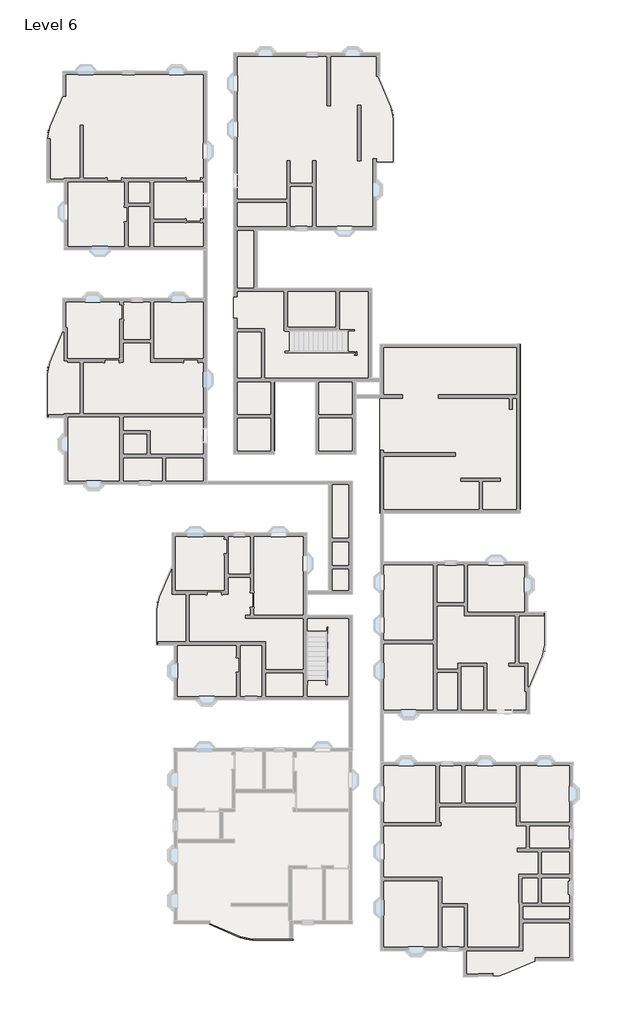
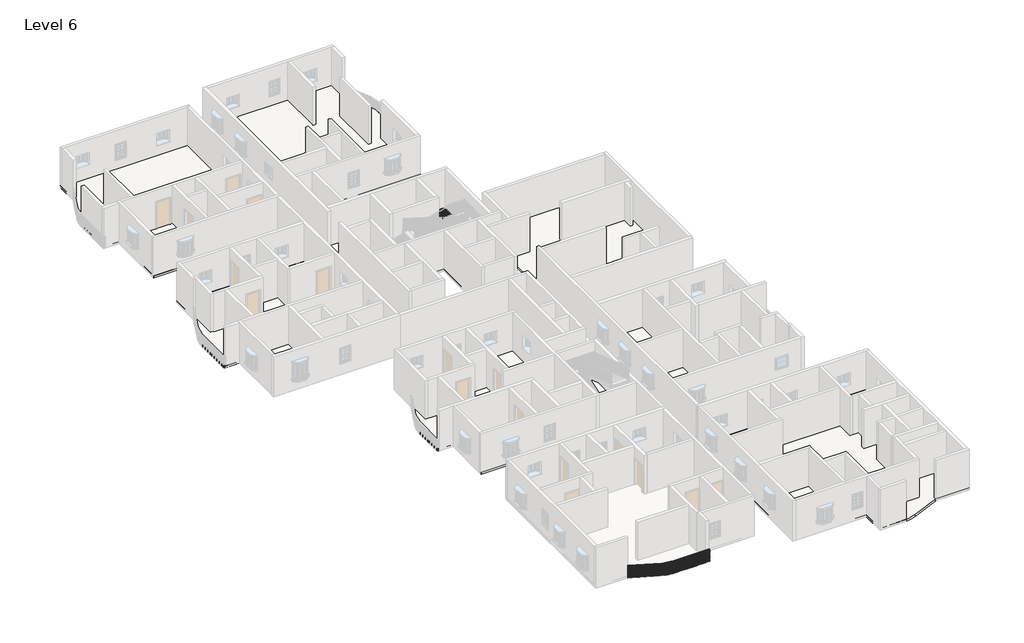
# One storey, part 5 of 14: 24 roofs, 1 railing.
"""IFC4 building model written with IfcOpenShell, lengths in millimetres."""

from ifc_helpers import new_model, si_unit, point, frame, frame_2d, origin, place, context, project, spatial, polyline, circle_curve, trimmed, segment, composite_curve, outline, extrude, element, save
from ifc_brep_helpers import plane_surface, cylinder_surface, revolved_surface, advanced_brep

model = new_model("IFC4")

# Units and contexts
model_context = context("Model", 3, world=origin())
ifc_project = project(units=[si_unit("LENGTHUNIT", "METRE", prefix="MILLI")], contexts=[model_context])

# Site, building, storey
site = spatial("IfcSite", under=ifc_project)
building = spatial("IfcBuilding", under=site)
storey = spatial("IfcBuildingStorey", under=building, Name="Level 6", Elevation=15240.0)

# Railing
placement = place(None, origin())
element("IfcRailing", 1, ObjectType="Handrail - Rectangular", at=placement, inside=storey, context=model_context, shape_type="SolidModel", body=[
    advanced_brep(
    [(-10014.8722294, -25076.9923935, 16154.4), (-10014.8722294, -25076.9923935, 16103.6), (-10034.8694485, -25123.6909077, 16103.6), (-10034.8694485, -25123.6909077, 16154.4), (-8065.5370278, -25911.7359335, 16154.4), (-8065.5370278, -25911.7359335, 16103.6), (-8085.5342469, -25958.4344477, 16103.6), (-8085.5342469, -25958.4344477, 16154.4), (-7315.6413127, -26065.5416506, 16103.6), (-7315.6413127, -26065.5416506, 16154.4), (-7315.6413127, -26116.3416506, 16103.6), (-7315.6413127, -26116.3416506, 16154.4), (-4746.0891351, -26065.5416506, 16154.4), (-4746.0891351, -26116.3416506, 16154.4), (-4746.0891351, -26116.3416506, 16103.6), (-4746.0891351, -26065.5416506, 16103.6)],
    [
        (0, 1),
        (1, 2),
        (2, 3),
        (3, 0),
        (0, 4),
        (4, 5),
        (5, 1),
        (5, 6),
        (6, 2),
        (6, 7),
        (7, 3),
        (7, 4),
        (8, 5, circle_curve(frame((-7315.6413127, -24160.5416506, 16103.6), z_axis=(0.0, 0.0, -1.0), x_axis=(-0.3936460446736572, -0.9192620907623599, 0.0)), 1905.0)),
        (4, 9, circle_curve(frame((-7315.6413127, -24160.5416506, 16154.4), z_axis=(0.0, 0.0, 1.0), x_axis=(-0.3936460446736572, -0.9192620907623599, 0.0)), 1905.0)),
        (9, 8),
        (10, 6, circle_curve(frame((-7315.6413127, -24160.5416506, 16103.6), z_axis=(0.0, 0.0, -1.0), x_axis=(-0.3936460446736572, -0.9192620907623599, 0.0)), 1955.8)),
        (8, 10),
        (11, 7, circle_curve(frame((-7315.6413127, -24160.5416506, 16154.4), z_axis=(0.0, 0.0, -1.0), x_axis=(-0.3936460446736572, -0.9192620907623599, 0.0)), 1955.8)),
        (10, 11),
        (11, 9),
        (12, 13),
        (13, 14),
        (14, 15),
        (15, 12),
        (9, 12),
        (15, 8),
        (14, 10),
        (13, 11),
    ],
    [
        plane_surface(frame((-10024.8708389, -25100.3416506, 16154.4), z_axis=(-0.9192620907623597, 0.39364604467365766, 0.0), x_axis=(0.39364604467365766, 0.9192620907623597, 0.0))),
        plane_surface(frame((-10014.8722294, -25076.9923935, 16154.4), z_axis=(0.3936460446736573, 0.9192620907623599, 0.0), x_axis=(0.9192620907623599, -0.3936460446736573, 0.0))),
        plane_surface(frame((-10014.8722294, -25076.9923935, 16103.6), z_axis=(0.0, 0.0, -1.0000000000000002), x_axis=(0.9192620907623599, -0.3936460446736573, 0.0))),
        plane_surface(frame((-10034.8694485, -25123.6909077, 16103.6), z_axis=(-0.39364604467365766, -0.9192620907623597, 0.0), x_axis=(0.9192620907623597, -0.39364604467365766, 0.0))),
        plane_surface(frame((-10034.8694485, -25123.6909077, 16154.4), z_axis=(0.0, 0.0, 1.0), x_axis=(0.9192620907623597, -0.39364604467365766, 0.0))),
        revolved_surface(polyline([(-8065.537027803317, -25911.735933502296, 16154.4), (-8065.537027803317, -25911.735933502296, 16103.6)]), (-7315.6413127, -24160.5416506, 16154.4), (0.0, 0.0, 1.0)),
        plane_surface(frame((-7315.6413127, -24160.5416506, 16103.6), z_axis=(0.0, 0.0, -1.0), x_axis=(-0.3936460446736572, -0.9192620907623599, 0.0))),
        cylinder_surface(frame((-7315.6413127, -24160.5416506, 16154.4), z_axis=(0.0, 0.0, 1.0), x_axis=(-0.3936460446736572, -0.9192620907623599, 0.0)), 1955.8),
        plane_surface(frame((-7315.6413127, -24160.5416506, 16154.4), z_axis=(0.0, 0.0, 1.0), x_axis=(-0.3936460446736572, -0.9192620907623599, 0.0))),
        plane_surface(frame((-4746.0891351, -26090.9416506, 16154.4), z_axis=(1.0, 0.0, 0.0), x_axis=(0.0, 1.0, 0.0))),
        plane_surface(frame((-7315.6413127, -26065.5416506, 16154.4), z_axis=(0.0, 1.0, 0.0), x_axis=(1.0, 0.0, 0.0))),
        plane_surface(frame((-7315.6413127, -26065.5416506, 16103.6), z_axis=(0.0, 0.0, -1.0), x_axis=(1.0, 0.0, 0.0))),
        plane_surface(frame((-7315.6413127, -26116.3416506, 16103.6), z_axis=(0.0, -1.0, 0.0), x_axis=(1.0, 0.0, 0.0))),
        plane_surface(frame((-7315.6413127, -26116.3416506, 16154.4), z_axis=(0.0, 0.0, 1.0), x_axis=(1.0, 0.0, 0.0))),
    ],
    [
        (0, [[1, 2, 3, 4]]),
        (1, [[-1, 5, 6, 7]]),
        (2, [[-2, -7, 8, 9]]),
        (3, [[-3, -9, 10, 11]]),
        (4, [[-4, -11, 12, -5]]),
        (5, [[13, -6, 14, 15]]),
        (6, [[16, -8, -13, 17]]),
        (7, [[18, -10, -16, 19]]),
        (8, [[-14, -12, -18, 20]]),
        (9, [[21, 22, 23, 24]]),
        (10, [[-15, 25, -24, 26]]),
        (11, [[-17, -26, -23, 27]]),
        (12, [[-19, -27, -22, 28]]),
        (13, [[-20, -28, -21, -25]]),
    ],
),
    extrude(outline(polyline([(-4785.1663127, -26100.4666506), (-4785.1663127, -26081.4166506), (-4766.1163127, -26081.4166506), (-4766.1163127, -26100.4666506), (-4785.1663127, -26100.4666506)])), frame((0.0, 0.0, 15240.0), z_axis=(0.0, 0.0, 1.0), x_axis=(1.0, 0.0, 0.0)), (0.0, 0.0, 1.0), 863.6),
    extrude(outline(polyline([(-4886.7663127, -26100.4666506), (-4886.7663127, -26081.4166506), (-4867.7163127, -26081.4166506), (-4867.7163127, -26100.4666506), (-4886.7663127, -26100.4666506)])), frame((0.0, 0.0, 15240.0), z_axis=(0.0, 0.0, 1.0), x_axis=(1.0, 0.0, 0.0)), (0.0, 0.0, 1.0), 863.6),
    extrude(outline(polyline([(-4988.3663127, -26100.4666506), (-4988.3663127, -26081.4166506), (-4969.3163127, -26081.4166506), (-4969.3163127, -26100.4666506), (-4988.3663127, -26100.4666506)])), frame((0.0, 0.0, 15240.0), z_axis=(0.0, 0.0, 1.0), x_axis=(1.0, 0.0, 0.0)), (0.0, 0.0, 1.0), 863.6),
    extrude(outline(polyline([(-5089.9663127, -26100.4666506), (-5089.9663127, -26081.4166506), (-5070.9163127, -26081.4166506), (-5070.9163127, -26100.4666506), (-5089.9663127, -26100.4666506)])), frame((0.0, 0.0, 15240.0), z_axis=(0.0, 0.0, 1.0), x_axis=(1.0, 0.0, 0.0)), (0.0, 0.0, 1.0), 863.6),
    extrude(outline(polyline([(-5191.5663127, -26100.4666506), (-5191.5663127, -26081.4166506), (-5172.5163127, -26081.4166506), (-5172.5163127, -26100.4666506), (-5191.5663127, -26100.4666506)])), frame((0.0, 0.0, 15240.0), z_axis=(0.0, 0.0, 1.0), x_axis=(1.0, 0.0, 0.0)), (0.0, 0.0, 1.0), 863.6),
    extrude(outline(polyline([(-5293.1663127, -26100.4666506), (-5293.1663127, -26081.4166506), (-5274.1163127, -26081.4166506), (-5274.1163127, -26100.4666506), (-5293.1663127, -26100.4666506)])), frame((0.0, 0.0, 15240.0), z_axis=(0.0, 0.0, 1.0), x_axis=(1.0, 0.0, 0.0)), (0.0, 0.0, 1.0), 863.6),
    extrude(outline(polyline([(-5394.7663127, -26100.4666506), (-5394.7663127, -26081.4166506), (-5375.7163127, -26081.4166506), (-5375.7163127, -26100.4666506), (-5394.7663127, -26100.4666506)])), frame((0.0, 0.0, 15240.0), z_axis=(0.0, 0.0, 1.0), x_axis=(1.0, 0.0, 0.0)), (0.0, 0.0, 1.0), 863.6),
    extrude(outline(polyline([(-5496.3663127, -26100.4666506), (-5496.3663127, -26081.4166506), (-5477.3163127, -26081.4166506), (-5477.3163127, -26100.4666506), (-5496.3663127, -26100.4666506)])), frame((0.0, 0.0, 15240.0), z_axis=(0.0, 0.0, 1.0), x_axis=(1.0, 0.0, 0.0)), (0.0, 0.0, 1.0), 863.6),
    extrude(outline(polyline([(-5597.9663127, -26100.4666506), (-5597.9663127, -26081.4166506), (-5578.9163127, -26081.4166506), (-5578.9163127, -26100.4666506), (-5597.9663127, -26100.4666506)])), frame((0.0, 0.0, 15240.0), z_axis=(0.0, 0.0, 1.0), x_axis=(1.0, 0.0, 0.0)), (0.0, 0.0, 1.0), 863.6),
    extrude(outline(polyline([(-5699.5663127, -26100.4666506), (-5699.5663127, -26081.4166506), (-5680.5163127, -26081.4166506), (-5680.5163127, -26100.4666506), (-5699.5663127, -26100.4666506)])), frame((0.0, 0.0, 15240.0), z_axis=(0.0, 0.0, 1.0), x_axis=(1.0, 0.0, 0.0)), (0.0, 0.0, 1.0), 863.6),
    extrude(outline(polyline([(-5801.1663127, -26100.4666506), (-5801.1663127, -26081.4166506), (-5782.1163127, -26081.4166506), (-5782.1163127, -26100.4666506), (-5801.1663127, -26100.4666506)])), frame((0.0, 0.0, 15240.0), z_axis=(0.0, 0.0, 1.0), x_axis=(1.0, 0.0, 0.0)), (0.0, 0.0, 1.0), 863.6),
    extrude(outline(polyline([(-5902.7663127, -26100.4666506), (-5902.7663127, -26081.4166506), (-5883.7163127, -26081.4166506), (-5883.7163127, -26100.4666506), (-5902.7663127, -26100.4666506)])), frame((0.0, 0.0, 15240.0), z_axis=(0.0, 0.0, 1.0), x_axis=(1.0, 0.0, 0.0)), (0.0, 0.0, 1.0), 863.6),
    extrude(outline(polyline([(-6004.3663127, -26100.4666506), (-6004.3663127, -26081.4166506), (-5985.3163127, -26081.4166506), (-5985.3163127, -26100.4666506), (-6004.3663127, -26100.4666506)])), frame((0.0, 0.0, 15240.0), z_axis=(0.0, 0.0, 1.0), x_axis=(1.0, 0.0, 0.0)), (0.0, 0.0, 1.0), 863.6),
    extrude(outline(polyline([(-6105.9663127, -26100.4666506), (-6105.9663127, -26081.4166506), (-6086.9163127, -26081.4166506), (-6086.9163127, -26100.4666506), (-6105.9663127, -26100.4666506)])), frame((0.0, 0.0, 15240.0), z_axis=(0.0, 0.0, 1.0), x_axis=(1.0, 0.0, 0.0)), (0.0, 0.0, 1.0), 863.6),
    extrude(outline(polyline([(-6207.5663127, -26100.4666506), (-6207.5663127, -26081.4166506), (-6188.5163127, -26081.4166506), (-6188.5163127, -26100.4666506), (-6207.5663127, -26100.4666506)])), frame((0.0, 0.0, 15240.0), z_axis=(0.0, 0.0, 1.0), x_axis=(1.0, 0.0, 0.0)), (0.0, 0.0, 1.0), 863.6),
    extrude(outline(polyline([(-6309.1663127, -26100.4666506), (-6309.1663127, -26081.4166506), (-6290.1163127, -26081.4166506), (-6290.1163127, -26100.4666506), (-6309.1663127, -26100.4666506)])), frame((0.0, 0.0, 15240.0), z_axis=(0.0, 0.0, 1.0), x_axis=(1.0, 0.0, 0.0)), (0.0, 0.0, 1.0), 863.6),
    extrude(outline(polyline([(-6410.7663127, -26100.4666506), (-6410.7663127, -26081.4166506), (-6391.7163127, -26081.4166506), (-6391.7163127, -26100.4666506), (-6410.7663127, -26100.4666506)])), frame((0.0, 0.0, 15240.0), z_axis=(0.0, 0.0, 1.0), x_axis=(1.0, 0.0, 0.0)), (0.0, 0.0, 1.0), 863.6),
    extrude(outline(polyline([(-6512.3663127, -26100.4666506), (-6512.3663127, -26081.4166506), (-6493.3163127, -26081.4166506), (-6493.3163127, -26100.4666506), (-6512.3663127, -26100.4666506)])), frame((0.0, 0.0, 15240.0), z_axis=(0.0, 0.0, 1.0), x_axis=(1.0, 0.0, 0.0)), (0.0, 0.0, 1.0), 863.6),
    extrude(outline(polyline([(-6613.9663127, -26100.4666506), (-6613.9663127, -26081.4166506), (-6594.9163127, -26081.4166506), (-6594.9163127, -26100.4666506), (-6613.9663127, -26100.4666506)])), frame((0.0, 0.0, 15240.0), z_axis=(0.0, 0.0, 1.0), x_axis=(1.0, 0.0, 0.0)), (0.0, 0.0, 1.0), 863.6),
    extrude(outline(polyline([(-6715.5663127, -26100.4666506), (-6715.5663127, -26081.4166506), (-6696.5163127, -26081.4166506), (-6696.5163127, -26100.4666506), (-6715.5663127, -26100.4666506)])), frame((0.0, 0.0, 15240.0), z_axis=(0.0, 0.0, 1.0), x_axis=(1.0, 0.0, 0.0)), (0.0, 0.0, 1.0), 863.6),
    extrude(outline(polyline([(-6817.1663127, -26100.4666506), (-6817.1663127, -26081.4166506), (-6798.1163127, -26081.4166506), (-6798.1163127, -26100.4666506), (-6817.1663127, -26100.4666506)])), frame((0.0, 0.0, 15240.0), z_axis=(0.0, 0.0, 1.0), x_axis=(1.0, 0.0, 0.0)), (0.0, 0.0, 1.0), 863.6),
    extrude(outline(polyline([(-6918.7663127, -26100.4666506), (-6918.7663127, -26081.4166506), (-6899.7163127, -26081.4166506), (-6899.7163127, -26100.4666506), (-6918.7663127, -26100.4666506)])), frame((0.0, 0.0, 15240.0), z_axis=(0.0, 0.0, 1.0), x_axis=(1.0, 0.0, 0.0)), (0.0, 0.0, 1.0), 863.6),
    extrude(outline(polyline([(-7020.3663127, -26100.4666506), (-7020.3663127, -26081.4166506), (-7001.3163127, -26081.4166506), (-7001.3163127, -26100.4666506), (-7020.3663127, -26100.4666506)])), frame((0.0, 0.0, 15240.0), z_axis=(0.0, 0.0, 1.0), x_axis=(1.0, 0.0, 0.0)), (0.0, 0.0, 1.0), 863.6),
    extrude(outline(polyline([(-7121.9663127, -26100.4666506), (-7121.9663127, -26081.4166506), (-7102.9163127, -26081.4166506), (-7102.9163127, -26100.4666506), (-7121.9663127, -26100.4666506)])), frame((0.0, 0.0, 15240.0), z_axis=(0.0, 0.0, 1.0), x_axis=(1.0, 0.0, 0.0)), (0.0, 0.0, 1.0), 863.6),
    extrude(outline(polyline([(-7223.5663127, -26100.4666506), (-7223.5663127, -26081.4166506), (-7204.5163127, -26081.4166506), (-7204.5163127, -26100.4666506), (-7223.5663127, -26100.4666506)])), frame((0.0, 0.0, 15240.0), z_axis=(0.0, 0.0, 1.0), x_axis=(1.0, 0.0, 0.0)), (0.0, 0.0, 1.0), 863.6),
    extrude(outline(polyline([(-7395.3185803, -26098.8530973), (-7394.6296262, -26079.8155596), (-7375.5920885, -26080.5045137), (-7376.2810426, -26099.5420514), (-7395.3185803, -26098.8530973)])), frame((0.0, 0.0, 15240.0), z_axis=(0.0, 0.0, 1.0), x_axis=(1.0, 0.0, 0.0)), (0.0, 0.0, 1.0), 863.6),
    extrude(outline(polyline([(-7497.177549, -26091.9774704), (-7495.4880357, -26073.0025384), (-7476.5131037, -26074.6920517), (-7478.2026169, -26093.6669837), (-7497.177549, -26091.9774704)])), frame((0.0, 0.0, 15240.0), z_axis=(0.0, 0.0, 1.0), x_axis=(1.0, 0.0, 0.0)), (0.0, 0.0, 1.0), 863.6),
    extrude(outline(polyline([(-7598.5337632, -26079.7528408), (-7595.8483698, -26060.8930645), (-7576.9885935, -26063.5784579), (-7579.6739869, -26082.4382342), (-7598.5337632, -26079.7528408)])), frame((0.0, 0.0, 15240.0), z_axis=(0.0, 0.0, 1.0), x_axis=(1.0, 0.0, 0.0)), (0.0, 0.0, 1.0), 863.6),
    extrude(outline(polyline([(-7699.1065227, -26062.2130639), (-7695.4326862, -26043.5206744), (-7676.7402967, -26047.1945108), (-7680.4141332, -26065.8869003), (-7699.1065227, -26062.2130639)])), frame((0.0, 0.0, 15240.0), z_axis=(0.0, 0.0, 1.0), x_axis=(1.0, 0.0, 0.0)), (0.0, 0.0, 1.0), 863.6),
    extrude(outline(polyline([(-7798.6172969, -26039.4067149), (-7793.9651918, -26020.9334797), (-7775.4919566, -26025.5855848), (-7780.1440617, -26044.05882), (-7798.6172969, -26039.4067149)])), frame((0.0, 0.0, 15240.0), z_axis=(0.0, 0.0, 1.0), x_axis=(1.0, 0.0, 0.0)), (0.0, 0.0, 1.0), 863.6),
    extrude(outline(polyline([(-7896.7904963, -26011.396955), (-7891.1730064, -25993.1940347), (-7872.9700861, -25998.8115246), (-7878.587576, -26017.0144449), (-7896.7904963, -26011.396955)])), frame((0.0, 0.0, 15240.0), z_axis=(0.0, 0.0, 1.0), x_axis=(1.0, 0.0, 0.0)), (0.0, 0.0, 1.0), 863.6),
    extrude(outline(polyline([(-7993.3542357, -25978.2613554), (-7986.7869183, -25960.379162), (-7968.9047249, -25966.9464794), (-7975.4720423, -25984.8286729), (-7993.3542357, -25978.2613554)])), frame((0.0, 0.0, 15240.0), z_axis=(0.0, 0.0, 1.0), x_axis=(1.0, 0.0, 0.0)), (0.0, 0.0, 1.0), 863.6),
    extrude(outline(polyline([(-8169.4357205, -25905.2369062), (-8161.9367633, -25887.7249634), (-8144.4248205, -25895.2239205), (-8151.9237777, -25912.7358634), (-8169.4357205, -25905.2369062)])), frame((0.0, 0.0, 15240.0), z_axis=(0.0, 0.0, 1.0), x_axis=(1.0, 0.0, 0.0)), (0.0, 0.0, 1.0), 863.6),
    extrude(outline(polyline([(-8262.8327489, -25865.2424681), (-8255.3337918, -25847.7305252), (-8237.8218489, -25855.2294824), (-8245.3208061, -25872.7414252), (-8262.8327489, -25865.2424681)])), frame((0.0, 0.0, 15240.0), z_axis=(0.0, 0.0, 1.0), x_axis=(1.0, 0.0, 0.0)), (0.0, 0.0, 1.0), 863.6),
    extrude(outline(polyline([(-8356.2297773, -25825.2480299), (-8348.7308202, -25807.7360871), (-8331.2188774, -25815.2350443), (-8338.7178345, -25832.7469871), (-8356.2297773, -25825.2480299)])), frame((0.0, 0.0, 15240.0), z_axis=(0.0, 0.0, 1.0), x_axis=(1.0, 0.0, 0.0)), (0.0, 0.0, 1.0), 863.6),
    extrude(outline(polyline([(-8449.6268058, -25785.2535918), (-8442.1278486, -25767.741649), (-8424.6159058, -25775.2406061), (-8432.1148629, -25792.752549), (-8449.6268058, -25785.2535918)])), frame((0.0, 0.0, 15240.0), z_axis=(0.0, 0.0, 1.0), x_axis=(1.0, 0.0, 0.0)), (0.0, 0.0, 1.0), 863.6),
    extrude(outline(polyline([(-8543.0238342, -25745.2591537), (-8535.524877, -25727.7472108), (-8518.0129342, -25735.246168), (-8525.5118914, -25752.7581108), (-8543.0238342, -25745.2591537)])), frame((0.0, 0.0, 15240.0), z_axis=(0.0, 0.0, 1.0), x_axis=(1.0, 0.0, 0.0)), (0.0, 0.0, 1.0), 863.6),
    extrude(outline(polyline([(-8636.4208626, -25705.2647155), (-8628.9219055, -25687.7527727), (-8611.4099626, -25695.2517298), (-8618.9089198, -25712.7636727), (-8636.4208626, -25705.2647155)])), frame((0.0, 0.0, 15240.0), z_axis=(0.0, 0.0, 1.0), x_axis=(1.0, 0.0, 0.0)), (0.0, 0.0, 1.0), 863.6),
    extrude(outline(polyline([(-8729.817891, -25665.2702774), (-8722.3189339, -25647.7583346), (-8704.806991, -25655.2572917), (-8712.3059482, -25672.7692345), (-8729.817891, -25665.2702774)])), frame((0.0, 0.0, 15240.0), z_axis=(0.0, 0.0, 1.0), x_axis=(1.0, 0.0, 0.0)), (0.0, 0.0, 1.0), 863.6),
    extrude(outline(polyline([(-8823.2149194, -25625.2758392), (-8815.7159623, -25607.7638964), (-8798.2040195, -25615.2628536), (-8805.7029766, -25632.7747964), (-8823.2149194, -25625.2758392)])), frame((0.0, 0.0, 15240.0), z_axis=(0.0, 0.0, 1.0), x_axis=(1.0, 0.0, 0.0)), (0.0, 0.0, 1.0), 863.6),
    extrude(outline(polyline([(-8916.6119479, -25585.2814011), (-8909.1129907, -25567.7694583), (-8891.6010479, -25575.2684154), (-8899.100005, -25592.7803583), (-8916.6119479, -25585.2814011)])), frame((0.0, 0.0, 15240.0), z_axis=(0.0, 0.0, 1.0), x_axis=(1.0, 0.0, 0.0)), (0.0, 0.0, 1.0), 863.6),
    extrude(outline(polyline([(-9010.0089763, -25545.286963), (-9002.5100191, -25527.7750201), (-8984.9980763, -25535.2739773), (-8992.4970335, -25552.7859201), (-9010.0089763, -25545.286963)])), frame((0.0, 0.0, 15240.0), z_axis=(0.0, 0.0, 1.0), x_axis=(1.0, 0.0, 0.0)), (0.0, 0.0, 1.0), 863.6),
    extrude(outline(polyline([(-9103.4060047, -25505.2925248), (-9095.9070476, -25487.780582), (-9078.3951047, -25495.2795391), (-9085.8940619, -25512.791482), (-9103.4060047, -25505.2925248)])), frame((0.0, 0.0, 15240.0), z_axis=(0.0, 0.0, 1.0), x_axis=(1.0, 0.0, 0.0)), (0.0, 0.0, 1.0), 863.6),
    extrude(outline(polyline([(-9196.8030331, -25465.2980867), (-9189.304076, -25447.7861439), (-9171.7921332, -25455.285101), (-9179.2910903, -25472.7970438), (-9196.8030331, -25465.2980867)])), frame((0.0, 0.0, 15240.0), z_axis=(0.0, 0.0, 1.0), x_axis=(1.0, 0.0, 0.0)), (0.0, 0.0, 1.0), 863.6),
    extrude(outline(polyline([(-9290.2000616, -25425.3036485), (-9282.7011044, -25407.7917057), (-9265.1891616, -25415.2906629), (-9272.6881187, -25432.8026057), (-9290.2000616, -25425.3036485)])), frame((0.0, 0.0, 15240.0), z_axis=(0.0, 0.0, 1.0), x_axis=(1.0, 0.0, 0.0)), (0.0, 0.0, 1.0), 863.6),
    extrude(outline(polyline([(-9383.59709, -25385.3092104), (-9376.0981328, -25367.7972676), (-9358.58619, -25375.2962247), (-9366.0851471, -25392.8081676), (-9383.59709, -25385.3092104)])), frame((0.0, 0.0, 15240.0), z_axis=(0.0, 0.0, 1.0), x_axis=(1.0, 0.0, 0.0)), (0.0, 0.0, 1.0), 863.6),
    extrude(outline(polyline([(-9476.9941184, -25345.3147723), (-9469.4951612, -25327.8028294), (-9451.9832184, -25335.3017866), (-9459.4821756, -25352.8137294), (-9476.9941184, -25345.3147723)])), frame((0.0, 0.0, 15240.0), z_axis=(0.0, 0.0, 1.0), x_axis=(1.0, 0.0, 0.0)), (0.0, 0.0, 1.0), 863.6),
    extrude(outline(polyline([(-9570.3911468, -25305.3203341), (-9562.8921897, -25287.8083913), (-9545.3802468, -25295.3073485), (-9552.879204, -25312.8192913), (-9570.3911468, -25305.3203341)])), frame((0.0, 0.0, 15240.0), z_axis=(0.0, 0.0, 1.0), x_axis=(1.0, 0.0, 0.0)), (0.0, 0.0, 1.0), 863.6),
    extrude(outline(polyline([(-9663.7881752, -25265.325896), (-9656.2892181, -25247.8139532), (-9638.7772753, -25255.3129103), (-9646.2762324, -25272.8248531), (-9663.7881752, -25265.325896)])), frame((0.0, 0.0, 15240.0), z_axis=(0.0, 0.0, 1.0), x_axis=(1.0, 0.0, 0.0)), (0.0, 0.0, 1.0), 863.6),
    extrude(outline(polyline([(-9757.1852037, -25225.3314579), (-9749.6862465, -25207.819515), (-9732.1743037, -25215.3184722), (-9739.6732608, -25232.830415), (-9757.1852037, -25225.3314579)])), frame((0.0, 0.0, 15240.0), z_axis=(0.0, 0.0, 1.0), x_axis=(1.0, 0.0, 0.0)), (0.0, 0.0, 1.0), 863.6),
    extrude(outline(polyline([(-9850.5822321, -25185.3370197), (-9843.0832749, -25167.8250769), (-9825.5713321, -25175.324034), (-9833.0702893, -25192.8359769), (-9850.5822321, -25185.3370197)])), frame((0.0, 0.0, 15240.0), z_axis=(0.0, 0.0, 1.0), x_axis=(1.0, 0.0, 0.0)), (0.0, 0.0, 1.0), 863.6),
    extrude(outline(polyline([(-9943.9792605, -25145.3425816), (-9936.4803034, -25127.8306387), (-9918.9683605, -25135.3295959), (-9926.4673177, -25152.8415387), (-9943.9792605, -25145.3425816)])), frame((0.0, 0.0, 15240.0), z_axis=(0.0, 0.0, 1.0), x_axis=(1.0, 0.0, 0.0)), (0.0, 0.0, 1.0), 863.6),
    extrude(outline(polyline([(-7325.1663127, -26100.4666506), (-7325.1663127, -26081.4166506), (-7306.1163127, -26081.4166506), (-7306.1163127, -26100.4666506), (-7325.1663127, -26100.4666506)])), frame((0.0, 0.0, 15240.0), z_axis=(0.0, 0.0, 1.0), x_axis=(1.0, 0.0, 0.0)), (0.0, 0.0, 1.0), 863.6),
    extrude(outline(polyline([(-8088.0410874, -25940.0916834), (-8080.5421302, -25922.5797406), (-8063.0301874, -25930.0786978), (-8070.5291445, -25947.5906406), (-8088.0410874, -25940.0916834)])), frame((0.0, 0.0, 15240.0), z_axis=(0.0, 0.0, 1.0), x_axis=(1.0, 0.0, 0.0)), (0.0, 0.0, 1.0), 863.6),
    extrude(outline(polyline([(-4765.1391351, -26100.4666506), (-4765.1391351, -26081.4166506), (-4746.0891351, -26081.4166506), (-4746.0891351, -26100.4666506), (-4765.1391351, -26100.4666506)])), frame((0.0, 0.0, 15240.0), z_axis=(0.0, 0.0, 1.0), x_axis=(1.0, 0.0, 0.0)), (0.0, 0.0, 1.0), 863.6),
    extrude(outline(polyline([(-10028.6203175, -25109.097622), (-10021.1213604, -25091.5856792), (-10003.6094175, -25099.0846363), (-10011.1083747, -25116.5965792), (-10028.6203175, -25109.097622)])), frame((0.0, 0.0, 15240.0), z_axis=(0.0, 0.0, 1.0), x_axis=(1.0, 0.0, 0.0)), (0.0, 0.0, 1.0), 863.6),
])

# Roofs
element("IfcRoof", 2, ObjectType="Generic - 12\"", at=placement, inside=storey, context=model_context, shape_type="SweptSolid", body=[
    extrude(outline(composite_curve([segment(polyline([(6070.4380523, -26783.9042694), (812.6380523, -26783.9042694), (812.6380523, -14845.9042694), (13017.3380523, -14845.9042694), (13017.3380523, -27431.6042694), (10660.5280667, -27431.6042694), (8711.1928652, -28266.3478094)]), True, "CONTINUOUS"), segment(trimmed(circle_curve(frame_2d((7951.2985405, -26491.8042694)), 1930.4), [point((8711.1928652, -28266.3478094))], [point((7953.0959373, -28422.2034326))], False, "CARTESIAN"), True, "CONTINUOUS"), segment(polyline([(7953.0959373, -28422.2034326), (6070.4380523, -28487.9472947), (6070.4380523, -26783.9042694)]), True, "CONTINUOUS")], self_intersect=False)), frame((0.0, 0.0, 15240.0), z_axis=(0.0, 0.0, 1.0), x_axis=(1.0, 0.0, 0.0)), (0.0, 0.0, 1.0), 152.4),
])
element("IfcRoof", 3, ObjectType="Generic - 12\"", at=placement, inside=storey, context=model_context, shape_type="SweptSolid", body=[
    extrude(outline(composite_curve([segment(polyline([(10274.1380523, -11759.8042694), (803.8108649, -11759.8042694), (803.8108649, -2133.2042694), (10159.8380523, -2133.2042694), (10159.8380523, -5352.6542694), (11264.7380523, -5352.6542694), (11264.7380523, -7397.5810633)]), True, "CONTINUOUS"), segment(trimmed(circle_curve(frame_2d((9334.3380523, -7397.5810633)), 1930.4), [point((11264.7380523, -7397.5810633))], [point((11108.8815923, -8157.475388))], False, "CARTESIAN"), True, "CONTINUOUS"), segment(polyline([(11108.8815923, -8157.475388), (10274.1380523, -10106.8105895), (10274.1380523, -11759.8042694)]), True, "CONTINUOUS")], self_intersect=False)), frame((0.0, 0.0, 15240.0), z_axis=(0.0, 0.0, 1.0), x_axis=(1.0, 0.0, 0.0)), (0.0, 0.0, 1.0), 152.4),
])
element("IfcRoof", 4, ObjectType="Generic - 12\"", at=placement, inside=storey, context=model_context, shape_type="SweptSolid", body=[
    extrude(outline(composite_curve([segment(polyline([(-13395.387215, -7421.9416506), (-13395.387215, -5140.4900045)]), True, "CONTINUOUS"), segment(trimmed(circle_curve(frame_2d((-11464.987215, -5140.4900045)), 1930.4), [point((-13395.387215, -5140.4900045))], [point((-13239.530755, -4380.5956799))], False, "CARTESIAN"), True, "CONTINUOUS"), segment(polyline([(-13239.530755, -4380.5956799), (-12404.787215, -2431.2604783), (-12404.787215, -322.6416506), (-3857.687215, -322.6416506), (-3857.687215, -5523.2916506), (-974.1891351, -5523.2916506), (-974.1891351, -10889.0416506), (-12290.487215, -10889.0416506), (-12290.487215, -7421.9416506), (-13395.387215, -7421.9416506)]), True, "CONTINUOUS")], self_intersect=False)), frame((0.0, 0.0, 15240.0), z_axis=(0.0, 0.0, 1.0), x_axis=(1.0, 0.0, 0.0)), (0.0, 0.0, 1.0), 152.4),
])
element("IfcRoof", 5, ObjectType="Generic - 12\"", at=placement, inside=storey, context=model_context, shape_type="SweptSolid", body=[
    extrude(outline(polyline([(-2472.7891351, 2953.9583494), (-961.4891351, 2953.9583494), (-961.4891351, -4202.4916506), (-2472.7891351, -4202.4916506), (-2472.7891351, 2953.9583494)])), frame((0.0, 0.0, 15240.0), z_axis=(0.0, 0.0, 1.0), x_axis=(1.0, 0.0, 0.0)), (0.0, 0.0, 1.0), 152.4),
])
element("IfcRoof", 6, ObjectType="Generic - 12\"", at=placement, inside=storey, context=model_context, shape_type="SweptSolid", body=[
    extrude(outline(composite_curve([segment(polyline([(-10194.3891351, 2750.7583494), (-19236.7891351, 2750.7583494), (-19236.7891351, 6979.8583494), (-20341.6891351, 6979.8583494), (-20341.6891351, 9746.7948172)]), True, "CONTINUOUS"), segment(trimmed(circle_curve(frame_2d((-18411.2891351, 9746.7948172)), 1930.4), [point((-20341.6891351, 9746.7948172))], [point((-20185.8326751, 10506.6891419))], False, "CARTESIAN"), True, "CONTINUOUS"), segment(polyline([(-20185.8326751, 10506.6891419), (-19351.0891351, 12456.0243434), (-19351.0891351, 14536.3583494), (-10194.3891351, 14536.3583494), (-10194.3891351, 2750.7583494)]), True, "CONTINUOUS")], self_intersect=False)), frame((0.0, 0.0, 15240.0), z_axis=(0.0, 0.0, 1.0), x_axis=(1.0, 0.0, 0.0)), (0.0, 0.0, 1.0), 152.4),
])
element("IfcRoof", 7, ObjectType="Generic - 12\"", at=placement, inside=storey, context=model_context, shape_type="SweptSolid", body=[
    extrude(outline(composite_curve([segment(polyline([(-10194.3891351, 17609.7583494), (-19236.7891351, 17609.7583494), (-19236.7891351, 21889.6583494), (-20341.6891351, 21889.6583494), (-20341.6891351, 24656.5948172)]), True, "CONTINUOUS"), segment(trimmed(circle_curve(frame_2d((-18411.2891351, 24656.5948172)), 1930.4), [point((-20341.6891351, 24656.5948172))], [point((-20185.8326751, 25416.4891419))], False, "CARTESIAN"), True, "CONTINUOUS"), segment(polyline([(-20185.8326751, 25416.4891419), (-19351.0891351, 27365.8243434), (-19351.0891351, 28950.8583494), (-10194.3891351, 28950.8583494), (-10194.3891351, 17609.7583494)]), True, "CONTINUOUS")], self_intersect=False)), frame((0.0, 0.0, 15240.0), z_axis=(0.0, 0.0, 1.0), x_axis=(1.0, 0.0, 0.0)), (0.0, 0.0, 1.0), 152.4),
])
element("IfcRoof", 8, ObjectType="Generic - 12\"", at=placement, inside=storey, context=model_context, shape_type="SweptSolid", body=[
    extrude(outline(composite_curve([segment(polyline([(-8492.5891351, 18875.1215905), (-8492.5891351, 30101.9215905), (664.1108649, 30101.9215905), (664.1108649, 28631.1875845), (1498.8544049, 26681.8523829)]), True, "CONTINUOUS"), segment(trimmed(circle_curve(frame_2d((-275.6891351, 25921.9580583)), 1930.4), [point((1498.8544049, 26681.8523829))], [point((1654.7108649, 25921.9580583))], False, "CARTESIAN"), True, "CONTINUOUS"), segment(polyline([(1654.7108649, 25921.9580583), (1654.7108649, 23155.0215905), (549.8108649, 23155.0215905), (549.8108649, 18875.1215905), (-8492.5891351, 18875.1215905)]), True, "CONTINUOUS")], self_intersect=False)), frame((0.0, 0.0, 15240.0), z_axis=(0.0, 0.0, 1.0), x_axis=(1.0, 0.0, 0.0)), (0.0, 0.0, 1.0), 152.4),
])
element("IfcRoof", 9, ObjectType="Generic - 12\"", at=placement, inside=storey, context=model_context, shape_type="SweptSolid", body=[
    extrude(outline(polyline([(-8492.5891351, 9478.4949943), (-5914.4891351, 9478.4949943), (-5914.4891351, 4665.1949943), (-8492.5891351, 4665.1949943), (-8492.5891351, 9478.4949943)])), frame((0.0, 0.0, 15240.0), z_axis=(0.0, 0.0, 1.0), x_axis=(1.0, 0.0, 0.0)), (0.0, 0.0, 1.0), 152.4),
])
element("IfcRoof", 10, ObjectType="Generic - 12\"", at=placement, inside=storey, context=model_context, shape_type="SweptSolid", body=[
    extrude(outline(polyline([(-3310.9891351, 9478.4949943), (-745.5891351, 9478.4949943), (-745.5891351, 4652.4949943), (-3310.9891351, 4652.4949943), (-3310.9891351, 9478.4949943)])), frame((0.0, 0.0, 15240.0), z_axis=(0.0, 0.0, 1.0), x_axis=(1.0, 0.0, 0.0)), (0.0, 0.0, 1.0), 152.4),
])
element("IfcRoof", 11, ObjectType="Generic - 12\"", at=placement, inside=storey, context=model_context, shape_type="SweptSolid", body=[
    extrude(outline(polyline([(-8492.5891351, 19078.3215905), (-6993.9891351, 19078.3215905), (-6993.9891351, 14988.9215905), (-8492.5891351, 14988.9215905), (-8492.5891351, 19078.3215905)])), frame((0.0, 0.0, 15240.0), z_axis=(0.0, 0.0, 1.0), x_axis=(1.0, 0.0, 0.0)), (0.0, 0.0, 1.0), 152.4),
])
element("IfcRoof", 12, ObjectType="Generic - 12\"", at=placement, inside=storey, context=model_context, shape_type="SweptSolid", body=[
    extrude(outline(polyline([(-8492.5891351, 15192.1215905), (257.7108649, 15192.1215905), (257.7108649, 9275.2949943), (-8492.5891351, 9275.2949943), (-8492.5891351, 15192.1215905)])), frame((0.0, 0.0, 15240.0), z_axis=(0.0, 0.0, 1.0), x_axis=(1.0, 0.0, 0.0)), (0.0, 0.0, 1.0), 152.4),
])
element("IfcRoof", 13, ObjectType="Generic - 12\"", at=placement, inside=storey, context=model_context, shape_type="SweptSolid", body=[
    extrude(outline(polyline([(793.5880523, 11646.2957306), (9677.2380523, 11646.2957306), (9677.2380523, 940.1957306), (793.5880523, 940.1957306), (793.5880523, 11646.2957306)])), frame((0.0, 0.0, 15240.0), z_axis=(0.0, 0.0, 1.0), x_axis=(1.0, 0.0, 0.0)), (0.0, 0.0, 1.0), 152.4),
])
element("IfcRoof", 14, ObjectType="Generic - 12\"", at=placement, inside=storey, context=model_context, shape_type="SweptSolid", body=[
    extrude(outline(composite_curve([segment(polyline([(6070.4380523, -26783.9042694), (812.6380523, -26783.9042694), (812.6380523, -14845.9042694), (13017.3380523, -14845.9042694), (13017.3380523, -27431.6042694), (10660.5280667, -27431.6042694), (8711.1928652, -28266.3478094)]), True, "CONTINUOUS"), segment(trimmed(circle_curve(frame_2d((7951.2985405, -26491.8042694)), 1930.4), [point((8711.1928652, -28266.3478094))], [point((7953.0959373, -28422.2034326))], False, "CARTESIAN"), True, "CONTINUOUS"), segment(polyline([(7953.0959373, -28422.2034326), (6070.4380523, -28487.9472947), (6070.4380523, -26783.9042694)]), True, "CONTINUOUS")], self_intersect=False)), frame((0.0, 0.0, 15240.0), z_axis=(0.0, 0.0, 1.0), x_axis=(1.0, 0.0, 0.0)), (0.0, 0.0, 1.0), 152.4),
])
element("IfcRoof", 15, ObjectType="Generic - 12\"", at=placement, inside=storey, context=model_context, shape_type="SweptSolid", body=[
    extrude(outline(composite_curve([segment(polyline([(10274.1380523, -11759.8042694), (803.8108649, -11759.8042694), (803.8108649, -2133.2042694), (10159.8380523, -2133.2042694), (10159.8380523, -5352.6542694), (11264.7380523, -5352.6542694), (11264.7380523, -7397.5810633)]), True, "CONTINUOUS"), segment(trimmed(circle_curve(frame_2d((9334.3380523, -7397.5810633)), 1930.4), [point((11264.7380523, -7397.5810633))], [point((11108.8815923, -8157.475388))], False, "CARTESIAN"), True, "CONTINUOUS"), segment(polyline([(11108.8815923, -8157.475388), (10274.1380523, -10106.8105895), (10274.1380523, -11759.8042694)]), True, "CONTINUOUS")], self_intersect=False)), frame((0.0, 0.0, 15240.0), z_axis=(0.0, 0.0, 1.0), x_axis=(1.0, 0.0, 0.0)), (0.0, 0.0, 1.0), 152.4),
])
element("IfcRoof", 16, ObjectType="Generic - 12\"", at=placement, inside=storey, context=model_context, shape_type="SweptSolid", body=[
    extrude(outline(composite_curve([segment(polyline([(-13395.387215, -7421.9416506), (-13395.387215, -5140.4900045)]), True, "CONTINUOUS"), segment(trimmed(circle_curve(frame_2d((-11464.987215, -5140.4900045)), 1930.4), [point((-13395.387215, -5140.4900045))], [point((-13239.530755, -4380.5956799))], False, "CARTESIAN"), True, "CONTINUOUS"), segment(polyline([(-13239.530755, -4380.5956799), (-12404.787215, -2431.2604783), (-12404.787215, -322.6416506), (-3857.687215, -322.6416506), (-3857.687215, -5523.2916506), (-974.1891351, -5523.2916506), (-974.1891351, -10889.0416506), (-12290.487215, -10889.0416506), (-12290.487215, -7421.9416506), (-13395.387215, -7421.9416506)]), True, "CONTINUOUS")], self_intersect=False)), frame((0.0, 0.0, 15240.0), z_axis=(0.0, 0.0, 1.0), x_axis=(1.0, 0.0, 0.0)), (0.0, 0.0, 1.0), 152.4),
])
element("IfcRoof", 17, ObjectType="Generic - 12\"", at=placement, inside=storey, context=model_context, shape_type="SweptSolid", body=[
    extrude(outline(polyline([(-2472.7891351, 2953.9583494), (-961.4891351, 2953.9583494), (-961.4891351, -4202.4916506), (-2472.7891351, -4202.4916506), (-2472.7891351, 2953.9583494)])), frame((0.0, 0.0, 15240.0), z_axis=(0.0, 0.0, 1.0), x_axis=(1.0, 0.0, 0.0)), (0.0, 0.0, 1.0), 152.4),
])
element("IfcRoof", 18, ObjectType="Generic - 12\"", at=placement, inside=storey, context=model_context, shape_type="SweptSolid", body=[
    extrude(outline(composite_curve([segment(polyline([(-10194.3891351, 2750.7583494), (-19236.7891351, 2750.7583494), (-19236.7891351, 6979.8583494), (-20341.6891351, 6979.8583494), (-20341.6891351, 9746.7948172)]), True, "CONTINUOUS"), segment(trimmed(circle_curve(frame_2d((-18411.2891351, 9746.7948172)), 1930.4), [point((-20341.6891351, 9746.7948172))], [point((-20185.8326751, 10506.6891419))], False, "CARTESIAN"), True, "CONTINUOUS"), segment(polyline([(-20185.8326751, 10506.6891419), (-19351.0891351, 12456.0243434), (-19351.0891351, 14536.3583494), (-10194.3891351, 14536.3583494), (-10194.3891351, 2750.7583494)]), True, "CONTINUOUS")], self_intersect=False)), frame((0.0, 0.0, 15240.0), z_axis=(0.0, 0.0, 1.0), x_axis=(1.0, 0.0, 0.0)), (0.0, 0.0, 1.0), 152.4),
])
element("IfcRoof", 19, ObjectType="Generic - 12\"", at=placement, inside=storey, context=model_context, shape_type="SweptSolid", body=[
    extrude(outline(composite_curve([segment(polyline([(-10194.3891351, 17609.7583494), (-19236.7891351, 17609.7583494), (-19236.7891351, 21889.6583494), (-20341.6891351, 21889.6583494), (-20341.6891351, 24656.5948172)]), True, "CONTINUOUS"), segment(trimmed(circle_curve(frame_2d((-18411.2891351, 24656.5948172)), 1930.4), [point((-20341.6891351, 24656.5948172))], [point((-20185.8326751, 25416.4891419))], False, "CARTESIAN"), True, "CONTINUOUS"), segment(polyline([(-20185.8326751, 25416.4891419), (-19351.0891351, 27365.8243434), (-19351.0891351, 28950.8583494), (-10194.3891351, 28950.8583494), (-10194.3891351, 17609.7583494)]), True, "CONTINUOUS")], self_intersect=False)), frame((0.0, 0.0, 15240.0), z_axis=(0.0, 0.0, 1.0), x_axis=(1.0, 0.0, 0.0)), (0.0, 0.0, 1.0), 152.4),
])
element("IfcRoof", 20, ObjectType="Generic - 12\"", at=placement, inside=storey, context=model_context, shape_type="SweptSolid", body=[
    extrude(outline(composite_curve([segment(polyline([(-8492.5891351, 18875.1215905), (-8492.5891351, 30101.9215905), (664.1108649, 30101.9215905), (664.1108649, 28631.1875845), (1498.8544049, 26681.8523829)]), True, "CONTINUOUS"), segment(trimmed(circle_curve(frame_2d((-275.6891351, 25921.9580583)), 1930.4), [point((1498.8544049, 26681.8523829))], [point((1654.7108649, 25921.9580583))], False, "CARTESIAN"), True, "CONTINUOUS"), segment(polyline([(1654.7108649, 25921.9580583), (1654.7108649, 23155.0215905), (549.8108649, 23155.0215905), (549.8108649, 18875.1215905), (-8492.5891351, 18875.1215905)]), True, "CONTINUOUS")], self_intersect=False)), frame((0.0, 0.0, 15240.0), z_axis=(0.0, 0.0, 1.0), x_axis=(1.0, 0.0, 0.0)), (0.0, 0.0, 1.0), 152.4),
])
element("IfcRoof", 21, ObjectType="Generic - 12\"", at=placement, inside=storey, context=model_context, shape_type="SweptSolid", body=[
    extrude(outline(polyline([(-8492.5891351, 9478.4949943), (-5914.4891351, 9478.4949943), (-5914.4891351, 4665.1949943), (-8492.5891351, 4665.1949943), (-8492.5891351, 9478.4949943)])), frame((0.0, 0.0, 15240.0), z_axis=(0.0, 0.0, 1.0), x_axis=(1.0, 0.0, 0.0)), (0.0, 0.0, 1.0), 152.4),
])
element("IfcRoof", 22, ObjectType="Generic - 12\"", at=placement, inside=storey, context=model_context, shape_type="SweptSolid", body=[
    extrude(outline(polyline([(-3310.9891351, 9478.4949943), (-745.5891351, 9478.4949943), (-745.5891351, 4652.4949943), (-3310.9891351, 4652.4949943), (-3310.9891351, 9478.4949943)])), frame((0.0, 0.0, 15240.0), z_axis=(0.0, 0.0, 1.0), x_axis=(1.0, 0.0, 0.0)), (0.0, 0.0, 1.0), 152.4),
])
element("IfcRoof", 23, ObjectType="Generic - 12\"", at=placement, inside=storey, context=model_context, shape_type="SweptSolid", body=[
    extrude(outline(polyline([(-8492.5891351, 19078.3215905), (-6993.9891351, 19078.3215905), (-6993.9891351, 14988.9215905), (-8492.5891351, 14988.9215905), (-8492.5891351, 19078.3215905)])), frame((0.0, 0.0, 15240.0), z_axis=(0.0, 0.0, 1.0), x_axis=(1.0, 0.0, 0.0)), (0.0, 0.0, 1.0), 152.4),
])
element("IfcRoof", 24, ObjectType="Generic - 12\"", at=placement, inside=storey, context=model_context, shape_type="SweptSolid", body=[
    extrude(outline(polyline([(-8492.5891351, 15192.1215905), (257.7108649, 15192.1215905), (257.7108649, 9275.2949943), (-8492.5891351, 9275.2949943), (-8492.5891351, 15192.1215905)])), frame((0.0, 0.0, 15240.0), z_axis=(0.0, 0.0, 1.0), x_axis=(1.0, 0.0, 0.0)), (0.0, 0.0, 1.0), 152.4),
])
element("IfcRoof", 25, ObjectType="Generic - 12\"", at=placement, inside=storey, context=model_context, shape_type="SweptSolid", body=[
    extrude(outline(polyline([(793.5880523, 11646.2957306), (9677.2380523, 11646.2957306), (9677.2380523, 940.1957306), (793.5880523, 940.1957306), (793.5880523, 11646.2957306)])), frame((0.0, 0.0, 15240.0), z_axis=(0.0, 0.0, 1.0), x_axis=(1.0, 0.0, 0.0)), (0.0, 0.0, 1.0), 152.4),
])

save(model, "model.ifc")

# Revit data of these elements
# Type "Handrail - Rectangular"
#   Assembly Code = "C2010400"
#   built-in parameter 1008612 = 0.0416667 (stored number, unit not read)
#   built-in parameter 1008611 = 0.0416667 (stored number, unit not read)
#   built-in parameter 1008609 = 0.333333 (stored number, unit not read)
#   built-in parameter 1008604 = 0.166667 (stored number, unit not read)
#   built-in parameter 1008603 = 0.166667 (stored number, unit not read)
#   Railing Height = 3' - 0"
#   built-in parameter 1008630 = 2
#   built-in parameter 1008610 = 2
#   built-in parameter 1008618 = Baluster - Square : 3/4"
# Type "Generic - 12\""
#   Assembly Code = "B1020"
#   Layers, outside or top first: 0' - 6" no material (function 1)
# Element 1 (IfcRailing, "Handrail - Rectangular")
#   Phase Created = New Construction
# Elements 2, 3, 4, 5, 6, 7, 8, 9, 10, 11, 12, 13, 14, 15, 16, 17, 18, 19, 21, 22, 24, 25 (IfcRoof, "Generic - 12\"")
#   built-in parameter 1001705 = 50.5 (stored number, unit not read)
#   built-in parameter 1001710 = 33615
#   Phase Created = New Construction
#   Materials on its faces: "Default Roof"
# Elements 20, 23 (IfcRoof, "Generic - 12\"")
#   built-in parameter 1001705 = 50.5 (stored number, unit not read)
#   built-in parameter 1001710 = 33615
#   Phase Created = New Construction
#   Materials on its faces: "Default Roof", "Wood - Stained"
# Materials
#   "Default Roof": colour RGB 88 101 114, transparency 0, Cost = 0
#   "Wood - Stained": class "Wood", colour RGB 224 178 126, transparency 0, Cost = 0
